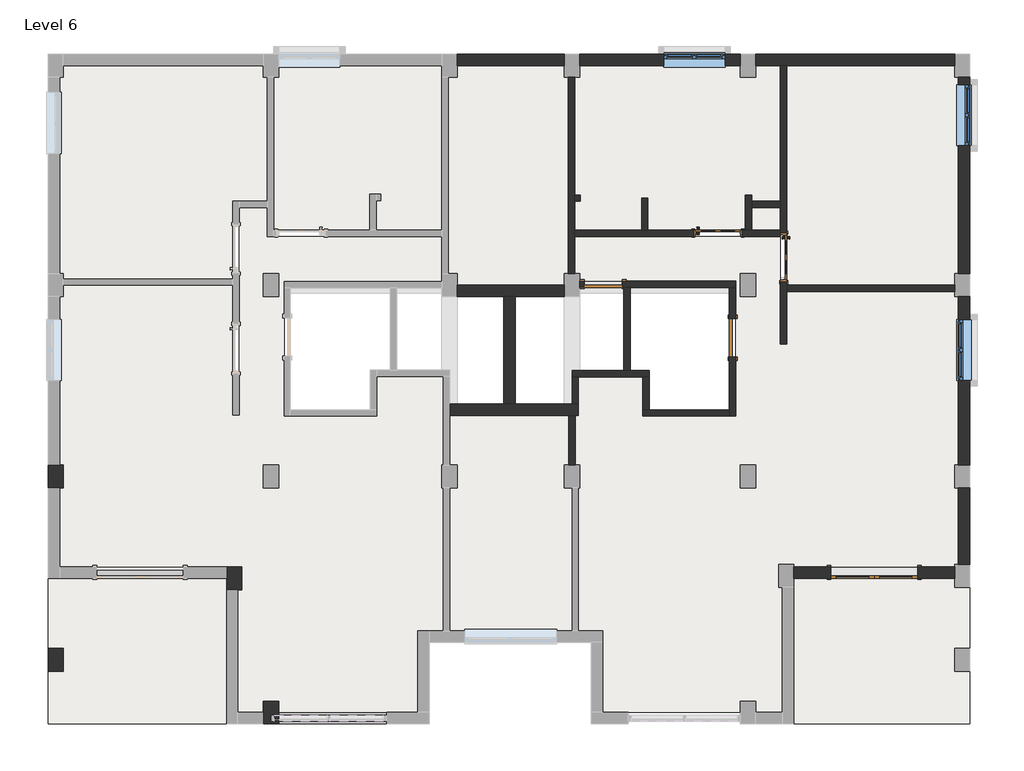
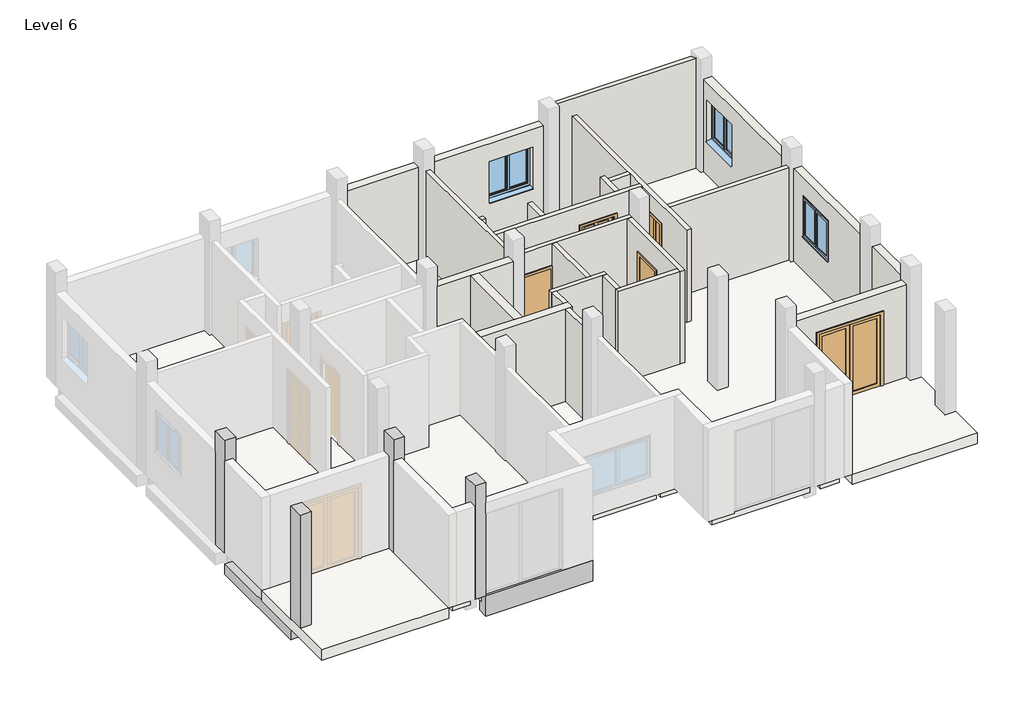
# One storey, part 2 of 3: 26 walls, 7 slabs, 5 doors, 4 columns, 3 beams, 3 windows.
"""IFC4 building model written with IfcOpenShell, lengths in millimetres."""

from ifc_helpers import new_model, si_unit, frame, origin, place, context, project, spatial, polyline, outline, extrude, faceted_brep, transform, mapped, element, save
from components import door_e52a3823, door_68a706ac, door_1fe7f57d, w2_0001_windows_4_x_4_9dec5fc7

model = new_model("IFC4")

# Units and contexts
model_context = context("Model", 3, world=origin())
ifc_project = project(units=[si_unit("LENGTHUNIT", "METRE", prefix="MILLI")], contexts=[model_context])

# Site, building, storey
site = spatial("IfcSite", under=ifc_project)
building = spatial("IfcBuilding", under=site)
storey = spatial("IfcBuildingStorey", under=building, Name="Level 6", Elevation=9448.8)

# Beams
placement = place(None, origin())
element("IfcBeam", 1, ObjectType="Concrete-Rectangular Beam : 12 x 24", at=placement, inside=storey, context=model_context, shape_type="Brep", body=[
    faceted_brep([(-9144.7786397, -9867.8620333, 8839.2), (-9144.7786397, -13068.2620333, 8839.2), (-9144.7786397, -13068.2620333, 9144.0), (-9144.7786397, -9867.8620333, 9144.0), (-8839.9786397, -9867.8620333, 8839.2), (-8839.9786397, -11518.8620333, 8839.2), (-8839.9786397, -11823.6620333, 8839.2), (-8839.9786397, -13068.2620333, 8839.2), (-8839.9786397, -9867.8620333, 9144.0), (-8839.9786397, -11518.8620333, 9144.0), (-8839.9786397, -11823.6620333, 9144.0), (-8839.9786397, -13068.2620333, 9144.0)], [[[0, 1, 2, 3]], [[1, 0, 4, 5, 6, 7]], [[7, 6, 5, 4, 8, 9, 10, 11]], [[4, 0, 3, 8]], [[1, 7, 11, 2]], [[3, 2, 11, 10, 9, 8]]]),
])
element("IfcBeam", 2, ObjectType="Concrete-Rectangular Beam : 12 x 24", at=placement, inside=storey, context=model_context, shape_type="SweptSolid", body=[
    extrude(outline(polyline([(-1550.9175798, -14272.0402089), (-1550.9175798, -14576.8402089), (-4548.1175798, -14576.8402089), (-4548.1175798, -14272.0402089), (-1550.9175798, -14272.0402089)])), frame((0.0, 0.0, 8839.2), z_axis=(0.0, 0.0, 1.0), x_axis=(1.0, 0.0, 0.0)), (0.0, 0.0, 1.0), 609.6),
])
element("IfcBeam", 3, ObjectType="Concrete-Rectangular Beam : 12 x 24", at=placement, inside=storey, context=model_context, shape_type="SweptSolid", body=[
    extrude(outline(polyline([(-8839.9786397, -11518.8620333), (-5589.5175798, -11518.8620333), (-5589.5175798, -11823.6620333), (-8839.9786397, -11823.6620333), (-8839.9786397, -11518.8620333)])), frame((0.0, 0.0, 8839.2), z_axis=(0.0, 0.0, 1.0), x_axis=(1.0, 0.0, 0.0)), (0.0, 0.0, 1.0), 304.8),
])

# Columns
element("IfcColumn", 4, ObjectType="Concrete-Rectangular-Column : 1'6\" X 1' COLUMN", at=placement, inside=storey, context=model_context, shape_type="Brep", body=[
    faceted_brep([(-8839.9786397, -9410.6620333, 9448.8), (-8839.9786397, -9867.8620333, 9448.8), (-9144.7786397, -9867.8620333, 9448.8), (-9144.7786397, -9410.6620333, 9448.8), (-8839.9786397, -9410.6620333, 12801.6), (-8839.9786397, -9867.8620333, 12801.6), (-8839.9786397, -9867.8620333, 9753.6), (-8839.9786397, -9410.6620333, 9753.6), (-9144.7786397, -9867.8620333, 12801.6), (-9144.7786397, -9867.8620333, 9753.6), (-9144.7786397, -9410.6620333, 12801.6), (-9144.7786397, -9410.6620333, 9753.6)], [[[0, 1, 2, 3]], [[4, 5, 6, 1, 0, 7]], [[5, 8, 9, 2, 1, 6]], [[8, 10, 11, 3, 2, 9]], [[10, 4, 7, 0, 3, 11]], [[4, 10, 8, 5]]]),
])
element("IfcColumn", 5, ObjectType="Concrete-Rectangular-Column : 1'6\" X 1' COLUMN", at=placement, inside=storey, context=model_context, shape_type="Brep", body=[
    faceted_brep([(-4548.1175798, -14119.6402089, 9448.8), (-4548.1175798, -14576.8402089, 9448.8), (-4852.9175798, -14576.8402089, 9448.8), (-4852.9175798, -14119.6402089, 9448.8), (-4548.1175798, -14119.6402089, 12801.6), (-4548.1175798, -14576.8402089, 12801.6), (-4548.1175798, -14119.6402089, 9753.6), (-4852.9175798, -14576.8402089, 12801.6), (-4852.9175798, -14119.6402089, 12801.6), (-4852.9175798, -14119.6402089, 9753.6)], [[[0, 1, 2, 3]], [[4, 5, 1, 0, 6]], [[5, 7, 2, 1]], [[7, 8, 9, 3, 2]], [[8, 4, 6, 0, 3, 9]], [[4, 8, 7, 5]]]),
])
element("IfcColumn", 6, ObjectType="Concrete-Rectangular-Column : 1'6\" X 1' COLUMN", at=placement, inside=storey, context=model_context, shape_type="Brep", body=[
    faceted_brep([(-8839.9786397, -13068.2620333, 9448.8), (-8839.9786397, -13525.4620333, 9448.8), (-9144.7786397, -13525.4620333, 9448.8), (-9144.7786397, -13068.2620333, 9448.8), (-8839.9786397, -13068.2620333, 12801.6), (-8839.9786397, -13525.4620333, 12801.6), (-8839.9786397, -13068.2620333, 9753.6), (-9144.7786397, -13525.4620333, 12801.6), (-9144.7786397, -13068.2620333, 12801.6), (-9144.7786397, -13068.2620333, 9753.6)], [[[0, 1, 2, 3]], [[4, 5, 1, 0, 6]], [[5, 7, 2, 1]], [[7, 8, 9, 3, 2]], [[8, 4, 6, 0, 3, 9]], [[4, 8, 7, 5]]]),
])
element("IfcColumn", 7, ObjectType="Concrete-Rectangular-Column : 1'6\" X 1' COLUMN", at=placement, inside=storey, context=model_context, shape_type="SweptSolid", body=[
    extrude(outline(polyline([(-5284.7175798, -11442.6620333), (-5284.7175798, -11899.8620333), (-5589.5175798, -11899.8620333), (-5589.5175798, -11442.6620333), (-5284.7175798, -11442.6620333)])), frame((0.0, 0.0, 9448.8), z_axis=(0.0, 0.0, 1.0), x_axis=(1.0, 0.0, 0.0)), (0.0, 0.0, 1.0), 3352.8),
])

# Doors
door_shape = door_e52a3823(model_context)
element("IfcDoor", 8, ObjectType="Door-Double-Glass : 68\" x 84\"", at=placement, inside=storey, context=model_context, shape_type="MappedRepresentation", body=[
    mapped(door_shape, transform((7313.6824202, -11554.5807833, 9448.8), x_axis=(-1.0, 0.0, 0.0), y_axis=(0.0, -1.0, 0.0), z_axis=(0.0, 0.0, 1.0))),
])
door_2_shape = door_68a706ac(model_context)
element("IfcDoor", 9, ObjectType="Door-Interior-Single-4_Panel-Wood : 36\" x 84\"", at=placement, inside=storey, context=model_context, shape_type="MappedRepresentation", body=[
    mapped(door_2_shape, transform((4202.1824202, -4789.1311634, 9448.8), x_axis=(1.0, 0.0, 0.0), y_axis=(0.0, 1.0, 0.0), z_axis=(0.0, 0.0, 1.0))),
])
element("IfcDoor", 10, ObjectType="Door-Interior-Single-4_Panel-Wood : 36\" x 84\"", at=placement, inside=storey, context=model_context, shape_type="MappedRepresentation", body=[
    mapped(door_2_shape, transform((5513.4574202, -5274.9061634, 9448.8), x_axis=(0.0, -1.0, 0.0), y_axis=(1.0, 0.0, 0.0), z_axis=(0.0, 0.0, 1.0))),
])
door_3_shape = door_1fe7f57d(model_context)
element("IfcDoor", 11, ObjectType="Single-Flush : 30\" x 80\"", at=placement, inside=storey, context=model_context, shape_type="MappedRepresentation", body=[
    mapped(door_3_shape, transform((1916.1824202, -5810.8691591, 9448.8), x_axis=(-1.0, 0.0, 0.0), y_axis=(0.0, -1.0, 0.0), z_axis=(0.0, 0.0, 1.0))),
])
element("IfcDoor", 12, ObjectType="Single-Flush : 30\" x 80\"", at=placement, inside=storey, context=model_context, shape_type="MappedRepresentation", body=[
    mapped(door_3_shape, transform((4494.2824202, -6877.6691591, 9448.8), x_axis=(0.0, 1.0, 0.0), y_axis=(-1.0, 0.0, 0.0), z_axis=(0.0, 0.0, 1.0))),
])

# Slabs
element("IfcSlab", 13, ObjectType="flooring 1'", at=placement, inside=storey, context=model_context, shape_type="SweptSolid", body=[
    extrude(outline(polyline([(-8916.1786397, -11442.6620333), (-8916.1786397, -9867.8620333), (-8839.9786397, -9867.8620333), (-8839.9786397, -9410.6620333), (-8916.1786397, -9410.6620333), (-8916.1786397, -6057.8620333), (-8839.9786397, -6057.8620333), (-8839.9786397, -5829.2620333), (-5462.5175798, -5829.2620333), (-5462.5175798, -8420.0620333), (-5335.5175798, -8420.0620333), (-5335.5175798, -4280.3104011), (-4776.7175798, -4280.3104011), (-4776.7175798, -4855.8061634), (-1296.9175798, -4855.8061634), (-1296.9175798, -5600.6620333), (-1296.9175798, -5758.8942903), (-4442.5950401, -5758.8942903), (-4442.5950401, -8439.1120333), (-2601.0950401, -8439.1120333), (-2601.0950401, -7651.7120333), (-1271.5175798, -7651.7120333), (-1271.5175798, -9410.6620333), (-1296.9175798, -9410.6620333), (-1296.9175798, -9867.8620333), (-1271.5175798, -9867.8620333), (-1271.5175798, -12722.6402089), (-1779.5175798, -12722.6402089), (-1779.5175798, -14348.2402089), (-4548.1175798, -14348.2402089), (-4548.1175798, -14119.6402089), (-4852.9175798, -14119.6402089), (-4852.9175798, -14348.2402089), (-5360.9175798, -14348.2402089), (-5360.9175798, -11899.8620333), (-5284.7175798, -11899.8620333), (-5284.7175798, -11442.6620333), (-5589.5175798, -11442.6620333), (-8916.1786397, -11442.6620333)])), frame((0.0, 0.0, 9144.0), z_axis=(0.0, 0.0, 1.0), x_axis=(1.0, 0.0, 0.0)), (0.0, 0.0, 1.0), 304.8),
])
element("IfcSlab", 14, ObjectType="flooring 1'", at=placement, inside=storey, context=model_context, shape_type="SweptSolid", body=[
    extrude(outline(polyline([(5446.7824202, -4855.8061634), (5446.7824202, -6583.0061634), (5573.7824202, -6583.0061634), (5573.7824202, -5956.2620333), (8913.8824202, -5956.2620333), (8913.8824202, -6057.8620333), (8990.0824202, -6057.8620333), (8990.0824202, -9410.6620333), (8913.8824202, -9410.6620333), (8913.8824202, -9867.8620333), (8990.0824202, -9867.8620333), (8990.0824202, -11391.8620333), (8913.8824202, -11391.8620333), (8913.8824202, -11442.6620333), (5713.4824202, -11442.6620333), (5713.4824202, -11391.8620333), (5408.6824202, -11391.8620333), (5408.6824202, -11849.0620333), (5484.8824202, -11849.0620333), (5484.8824202, -14348.2402089), (4951.4824202, -14348.2402089), (4951.4824202, -14119.6402089), (4646.6824202, -14119.6402089), (4646.6824202, -14348.2402089), (1903.4824202, -14348.2402089), (1903.4824202, -12722.6402089), (1420.8824202, -12722.6402089), (1420.8824202, -9867.8620333), (1446.2824202, -9867.8620333), (1446.2824202, -9410.6620333), (1357.3824202, -9410.6620333), (1357.3824202, -8426.4120333), (1420.8824202, -8426.4120333), (1420.8824202, -7660.8890971), (2703.5824202, -7660.8890971), (2703.5824202, -8439.7691591), (4557.7824202, -8439.7691591), (4557.7824202, -5747.3691591), (1446.2824202, -5747.3691591), (1446.2824202, -5600.6620333), (1344.6824202, -5600.6620333), (1344.6824202, -4855.8061634), (5446.7824202, -4855.8061634)])), frame((0.0, 0.0, 9144.0), z_axis=(0.0, 0.0, 1.0), x_axis=(1.0, 0.0, 0.0)), (0.0, 0.0, 1.0), 304.8),
])
element("IfcSlab", 15, ObjectType="flooring 1'", at=placement, inside=storey, context=model_context, shape_type="SweptSolid", body=[
    extrude(outline(polyline([(-8839.9786397, -1680.8061634), (-8839.9786397, -1452.2061634), (-4852.9175798, -1452.2061634), (-4852.9175798, -1680.8061634), (-4776.7175798, -1680.8061634), (-4776.7175798, -4153.3104011), (-5462.5175798, -4153.3104011), (-5462.5175798, -5702.2620333), (-8839.9786397, -5702.2620333), (-8839.9786397, -5600.6620333), (-8916.1786397, -5600.6620333), (-8916.1786397, -1680.8061634), (-8839.9786397, -1680.8061634)])), frame((0.0, 0.0, 9144.0), z_axis=(0.0, 0.0, 1.0), x_axis=(1.0, 0.0, 0.0)), (0.0, 0.0, 1.0), 304.8),
    extrude(outline(polyline([(-2732.0175798, -4728.8061634), (-4649.7175798, -4728.8061634), (-4649.7175798, -1680.8061634), (-4548.1175798, -1680.8061634), (-4548.1175798, -1452.2061634), (-1296.9175798, -1452.2061634), (-1296.9175798, -4728.8061634), (-2605.0175798, -4728.8061634), (-2605.0175798, -4144.6061634), (-2516.1175798, -4144.6061634), (-2516.1175798, -4017.6061634), (-2732.0175798, -4017.6061634), (-2732.0175798, -4728.8061634)])), frame((0.0, 0.0, 9144.0), z_axis=(0.0, 0.0, 1.0), x_axis=(1.0, 0.0, 0.0)), (0.0, 0.0, 1.0), 304.8),
])
element("IfcSlab", 16, ObjectType="flooring 1'", at=placement, inside=storey, context=model_context, shape_type="SweptSolid", body=[
    extrude(outline(polyline([(4646.6824202, -1452.2061634), (4646.6824202, -1680.8061634), (4951.4824202, -1680.8061634), (4951.4824202, -1452.2061634), (5446.7824202, -1452.2061634), (5446.7824202, -4157.3061634), (4875.2824202, -4157.3061634), (4875.2824202, -4030.3061634), (4748.2824202, -4030.3061634), (4748.2824202, -4728.8061634), (2805.1824202, -4728.8061634), (2805.1824202, -4093.8061634), (2678.1824202, -4093.8061634), (2678.1824202, -4728.8061634), (1344.6824202, -4728.8061634), (1344.6824202, -4157.3061634), (1458.9824202, -4157.3061634), (1458.9824202, -4030.3061634), (1344.6824202, -4030.3061634), (1344.6824202, -1680.8061634), (1446.2824202, -1680.8061634), (1446.2824202, -1452.2061634), (4646.6824202, -1452.2061634)])), frame((0.0, 0.0, 9144.0), z_axis=(0.0, 0.0, 1.0), x_axis=(1.0, 0.0, 0.0)), (0.0, 0.0, 1.0), 304.8),
    extrude(outline(polyline([(5446.7824202, -4284.3061634), (5446.7824202, -4728.8061634), (4875.2824202, -4728.8061634), (4875.2824202, -4284.3061634), (5446.7824202, -4284.3061634)])), frame((0.0, 0.0, 9144.0), z_axis=(0.0, 0.0, 1.0), x_axis=(1.0, 0.0, 0.0)), (0.0, 0.0, 1.0), 304.8),
    extrude(outline(polyline([(8913.8824202, -5829.2620333), (5573.7824202, -5829.2620333), (5573.7824202, -1452.2061634), (8913.8824202, -1452.2061634), (8913.8824202, -1680.8061634), (8990.0824202, -1680.8061634), (8990.0824202, -5600.6620333), (8913.8824202, -5600.6620333), (8913.8824202, -5829.2620333)])), frame((0.0, 0.0, 9144.0), z_axis=(0.0, 0.0, 1.0), x_axis=(1.0, 0.0, 0.0)), (0.0, 0.0, 1.0), 304.8),
])
element("IfcSlab", 17, ObjectType="flooring 1'", at=placement, inside=storey, context=model_context, shape_type="SweptSolid", body=[
    extrude(outline(polyline([(1141.4824202, -1452.2061634), (1141.4824202, -1680.8061634), (1217.6824202, -1680.8061634), (1217.6824202, -5600.6620333), (1141.4824202, -5600.6620333), (1141.4824202, -5829.2620333), (-992.1175798, -5829.2620333), (-992.1175798, -5600.6620333), (-1169.9175798, -5600.6620333), (-1169.9175798, -1680.8061634), (-992.1175798, -1680.8061634), (-992.1175798, -1452.2061634), (1141.4824202, -1452.2061634)])), frame((0.0, 0.0, 9144.0), z_axis=(0.0, 0.0, 1.0), x_axis=(1.0, 0.0, 0.0)), (0.0, 0.0, 1.0), 304.8),
])
element("IfcSlab", 18, ObjectType="flooring 1'", at=placement, inside=storey, context=model_context, shape_type="SweptSolid", body=[
    extrude(outline(polyline([(1293.8824202, -12722.6402089), (-1144.5175798, -12722.6402089), (-1144.5175798, -9867.8620333), (-992.1175798, -9867.8620333), (-992.1175798, -9410.6620333), (-1144.5175798, -9410.6620333), (-1144.5175798, -8426.4120333), (1230.3824202, -8426.4120333), (1230.3824202, -9410.6620333), (1141.4824202, -9410.6620333), (1141.4824202, -9867.8620333), (1293.8824202, -9867.8620333), (1293.8824202, -12722.6402089)])), frame((0.0, 0.0, 9144.0), z_axis=(0.0, 0.0, 1.0), x_axis=(1.0, 0.0, 0.0)), (0.0, 0.0, 1.0), 304.8),
])
element("IfcSlab", 19, ObjectType="flooring 1'", at=placement, inside=storey, context=model_context, shape_type="SweptSolid", body=[
    extrude(outline(polyline([(-5589.5175798, -11671.2620333), (-5589.5175798, -14576.8402089), (-9144.7786397, -14576.8402089), (-9144.7786397, -11671.2620333), (-5589.5175798, -11671.2620333)])), frame((0.0, 0.0, 9144.0), z_axis=(0.0, 0.0, 1.0), x_axis=(1.0, 0.0, 0.0)), (0.0, 0.0, 1.0), 304.8),
    extrude(outline(polyline([(9218.6824202, -11671.2620333), (9218.6824202, -14576.8402089), (5713.4824202, -14576.8402089), (5713.4824202, -11671.2620333), (9218.6824202, -11671.2620333)])), frame((0.0, 0.0, 9144.0), z_axis=(0.0, 0.0, 1.0), x_axis=(1.0, 0.0, 0.0)), (0.0, 0.0, 1.0), 304.8),
])

# Walls
element("IfcWall", 20, ObjectType="EXTERIOR WALL 9\"", at=placement, inside=storey, context=model_context, shape_type="SweptSolid", body=[
    extrude(outline(polyline([(1141.4824202, -1452.2061634), (-992.1175798, -1452.2061634), (-992.1175798, -1223.6061634), (1141.4824202, -1223.6061634), (1141.4824202, -1452.2061634)])), frame((0.0, 0.0, 9448.8), z_axis=(0.0, 0.0, 1.0), x_axis=(1.0, 0.0, 0.0)), (0.0, 0.0, 1.0), 2743.2),
])
element("IfcWall", 21, ObjectType="EXTERIOR WALL 9\"", at=placement, inside=storey, context=model_context, shape_type="SweptSolid", body=[
    extrude(outline(polyline([(9448.8, 1446.2824202), (9448.8, 4646.6824202), (12192.0, 4646.6824202), (12192.0, 1446.2824202), (9448.8, 1446.2824202)]), holes=[polyline([(10448.8, 4341.8824202), (10448.8, 3122.6824202), (11668.0, 3122.6824202), (11668.0, 4341.8824202), (10448.8, 4341.8824202)])]), frame((0.0, -1452.2061634, 0.0), z_axis=(0.0, 1.0, 0.0), x_axis=(0.0, 0.0, 1.0)), (0.0, 0.0, 1.0), 228.6),
])
element("IfcWall", 22, ObjectType="EXTERIOR WALL 9\"", at=placement, inside=storey, context=model_context, shape_type="Brep", body=[
    faceted_brep([(4951.4824202, -1452.2061634, 9448.8), (5446.7824202, -1452.2061634, 9448.8), (5573.7824202, -1452.2061634, 9448.8), (8913.8824202, -1452.2061634, 9448.8), (8913.8824202, -1452.2061634, 12704.6626409), (4951.4824202, -1452.2061634, 12704.6626409), (4951.4824202, -1223.6061634, 9448.8), (4951.4824202, -1223.6061634, 12615.578652), (8913.8824202, -1223.6061634, 12615.578652), (8913.8824202, -1223.6061634, 9448.8)], [[[0, 1, 2, 3, 4, 5]], [[6, 7, 8, 9]], [[3, 2, 1, 0, 6, 9]], [[4, 3, 9, 8]], [[0, 5, 7, 6]], [[5, 4, 8, 7]]]),
])
element("IfcWall", 23, ObjectType="EXTERIOR WALL 9\"", at=placement, inside=storey, context=model_context, shape_type="SweptSolid", body=[
    extrude(outline(polyline([(-1680.8061634, 9448.8), (-5600.6620333, 9448.8), (-5600.6620333, 12192.0), (-1680.8061634, 12192.0), (-1680.8061634, 9448.8)]), holes=[polyline([(-3052.4061634, 10448.8), (-1833.2061634, 10448.8), (-1833.2061634, 11668.0), (-3052.4061634, 11668.0), (-3052.4061634, 10448.8)])]), frame((8990.0824202, 0.0, 0.0), z_axis=(1.0, 0.0, 0.0), x_axis=(0.0, 1.0, 0.0)), (0.0, 0.0, 1.0), 228.6),
])
element("IfcWall", 24, ObjectType="EXTERIOR WALL 9\"", at=placement, inside=storey, context=model_context, shape_type="SweptSolid", body=[
    extrude(outline(polyline([(-6057.8620333, 9448.8), (-9410.6620333, 9448.8), (-9410.6620333, 12192.0), (-6057.8620333, 12192.0), (-6057.8620333, 9448.8)]), holes=[polyline([(-6515.0620333, 10448.8), (-6515.0620333, 11668.0), (-7734.2620333, 11668.0), (-7734.2620333, 10448.8), (-6515.0620333, 10448.8)])]), frame((8990.0824202, 0.0, 0.0), z_axis=(1.0, 0.0, 0.0), x_axis=(0.0, 1.0, 0.0)), (0.0, 0.0, 1.0), 228.6),
])
element("IfcWall", 25, ObjectType="EXTERIOR WALL 9\"", at=placement, inside=storey, context=model_context, shape_type="SweptSolid", body=[
    extrude(outline(polyline([(8990.0824202, -11391.8620333), (8990.0824202, -9867.8620333), (9218.6824202, -9867.8620333), (9218.6824202, -11391.8620333), (8990.0824202, -11391.8620333)])), frame((0.0, 0.0, 9448.8), z_axis=(0.0, 0.0, 1.0), x_axis=(1.0, 0.0, 0.0)), (0.0, 0.0, 1.0), 2743.2),
])
element("IfcWall", 26, ObjectType="EXTERIOR WALL 9\"", at=placement, inside=storey, context=model_context, shape_type="SweptSolid", body=[
    extrude(outline(polyline([(12192.0, 5713.4824202), (9448.8, 5713.4824202), (9448.8, 6450.0824202), (11582.4, 6450.0824202), (11582.4, 8177.2824202), (9448.8, 8177.2824202), (9448.8, 8913.8824202), (12192.0, 8913.8824202), (12192.0, 5713.4824202)])), frame((0.0, -11671.2620333, 0.0), z_axis=(0.0, 1.0, 0.0), x_axis=(0.0, 0.0, 1.0)), (0.0, 0.0, 1.0), 228.6),
])
element("IfcWall", 27, ObjectType="EXTERIOR WALL 9\"", at=placement, inside=storey, context=model_context, shape_type="Brep", body=[
    faceted_brep([(1141.4824202, -5829.2620333, 9448.8), (-992.1175798, -5829.2620333, 9448.8), (-992.1175798, -5829.2620333, 12192.0), (1141.4824202, -5829.2620333, 12192.0), (1141.4824202, -6057.8620333, 9448.8), (1141.4824202, -6057.8620333, 12192.0), (163.5824202, -6057.8620333, 12192.0), (-65.0175798, -6057.8620333, 12192.0), (-992.1175798, -6057.8620333, 12192.0), (-992.1175798, -6057.8620333, 9448.8), (-65.0175798, -6057.8620333, 9448.8), (163.5824202, -6057.8620333, 9448.8)], [[[0, 1, 2, 3]], [[4, 5, 6, 7, 8, 9, 10, 11]], [[1, 0, 4, 11, 10, 9]], [[2, 1, 9, 8]], [[3, 2, 8, 7, 6, 5]], [[0, 3, 5, 4]]]),
])
element("IfcWall", 28, ObjectType="EXTERIOR WALL 9\"", at=placement, inside=storey, context=model_context, shape_type="SweptSolid", body=[
    extrude(outline(polyline([(-65.0175798, -8197.8120333), (-65.0175798, -6057.8620333), (163.5824202, -6057.8620333), (163.5824202, -8197.8120333), (-65.0175798, -8197.8120333)])), frame((0.0, 0.0, 9448.8), z_axis=(0.0, 0.0, 1.0), x_axis=(1.0, 0.0, 0.0)), (0.0, 0.0, 1.0), 2743.2),
])
element("IfcWall", 29, ObjectType="EXTERIOR WALL 9\"", at=placement, inside=storey, context=model_context, shape_type="Brep", body=[
    faceted_brep([(-1144.5175798, -8426.4120333, 9448.8), (1230.3824202, -8426.4120333, 9448.8), (1357.3824202, -8426.4120333, 9448.8), (1420.8824202, -8426.4120333, 9448.8), (1420.8824202, -8426.4120333, 12192.0), (1357.3824202, -8426.4120333, 12192.0), (1230.3824202, -8426.4120333, 12192.0), (-1144.5175798, -8426.4120333, 12192.0), (-1144.5175798, -8197.8120333, 9448.8), (-1144.5175798, -8197.8120333, 12192.0), (-65.0175798, -8197.8120333, 12192.0), (163.5824202, -8197.8120333, 12192.0), (1293.8824202, -8197.8120333, 12192.0), (1420.8824202, -8197.8120333, 12192.0), (1420.8824202, -8197.8120333, 9448.8), (1293.8824202, -8197.8120333, 9448.8), (163.5824202, -8197.8120333, 9448.8), (-65.0175798, -8197.8120333, 9448.8)], [[[0, 1, 2, 3, 4, 5, 6, 7]], [[8, 9, 10, 11, 12, 13, 14, 15, 16, 17]], [[3, 2, 1, 0, 8, 17, 16, 15, 14]], [[7, 6, 5, 4, 13, 12, 11, 10, 9]], [[0, 7, 9, 8]], [[4, 3, 14, 13]]]),
])
element("IfcWall", 30, ObjectType="INTERIOR WALL 5\"", at=placement, inside=storey, context=model_context, shape_type="Brep", body=[
    faceted_brep([(1217.6824202, -1680.8061634, 9448.8), (1217.6824202, -5600.6620333, 9448.8), (1217.6824202, -5600.6620333, 12192.0), (1217.6824202, -1680.8061634, 12192.0), (1344.6824202, -1680.8061634, 9448.8), (1344.6824202, -1680.8061634, 12192.0), (1344.6824202, -4030.3061634, 12192.0), (1344.6824202, -4157.3061634, 12192.0), (1344.6824202, -4728.8061634, 12192.0), (1344.6824202, -4855.8061634, 12192.0), (1344.6824202, -5600.6620333, 12192.0), (1344.6824202, -5600.6620333, 9448.8), (1344.6824202, -4855.8061634, 9448.8), (1344.6824202, -4728.8061634, 9448.8), (1344.6824202, -4157.3061634, 9448.8), (1344.6824202, -4030.3061634, 9448.8)], [[[0, 1, 2, 3]], [[4, 5, 6, 7, 8, 9, 10, 11, 12, 13, 14, 15]], [[1, 0, 4, 15, 14, 13, 12, 11]], [[2, 1, 11, 10]], [[3, 2, 10, 9, 8, 7, 6, 5]], [[0, 3, 5, 4]]]),
])
element("IfcWall", 31, ObjectType="INTERIOR WALL 5\"", at=placement, inside=storey, context=model_context, shape_type="Brep", body=[
    faceted_brep([(5446.7824202, -4855.8061634, 12192.0), (1344.6824202, -4855.8061634, 12192.0), (1344.6824202, -4855.8061634, 9448.8), (3719.5824202, -4855.8061634, 9448.8), (3719.5824202, -4855.8061634, 11607.8), (4684.7824202, -4855.8061634, 11607.8), (4684.7824202, -4855.8061634, 9448.8), (5446.7824202, -4855.8061634, 9448.8), (1344.6824202, -4728.8061634, 12192.0), (2678.1824202, -4728.8061634, 12192.0), (2805.1824202, -4728.8061634, 12192.0), (4748.2824202, -4728.8061634, 12192.0), (4875.2824202, -4728.8061634, 12192.0), (5446.7824202, -4728.8061634, 12192.0), (5446.7824202, -4728.8061634, 9448.8), (4875.2824202, -4728.8061634, 9448.8), (4748.2824202, -4728.8061634, 9448.8), (4684.7824202, -4728.8061634, 9448.8), (4684.7824202, -4728.8061634, 11607.8), (3719.5824202, -4728.8061634, 11607.8), (3719.5824202, -4728.8061634, 9448.8), (2805.1824202, -4728.8061634, 9448.8), (2678.1824202, -4728.8061634, 9448.8), (1344.6824202, -4728.8061634, 9448.8)], [[[0, 1, 2, 3, 4, 5, 6, 7]], [[8, 9, 10, 11, 12, 13, 14, 15, 16, 17, 18, 19, 20, 21, 22, 23]], [[2, 23, 22, 21, 20, 3]], [[14, 7, 6, 17, 16, 15]], [[1, 0, 13, 12, 11, 10, 9, 8]], [[2, 1, 8, 23]], [[0, 7, 14, 13]], [[5, 18, 17, 6]], [[18, 5, 4, 19]], [[19, 4, 3, 20]]]),
])
element("IfcWall", 32, ObjectType="INTERIOR WALL 5\"", at=placement, inside=storey, context=model_context, shape_type="Brep", body=[
    faceted_brep([(4875.2824202, -4728.8061634, 9448.8), (4875.2824202, -4284.3061634, 9448.8), (4875.2824202, -4157.3061634, 9448.8), (4875.2824202, -4030.3061634, 9448.8), (4875.2824202, -4030.3061634, 12192.0), (4875.2824202, -4157.3061634, 12192.0), (4875.2824202, -4284.3061634, 12192.0), (4875.2824202, -4728.8061634, 12192.0), (4748.2824202, -4728.8061634, 9448.8), (4748.2824202, -4728.8061634, 12192.0), (4748.2824202, -4030.3061634, 12192.0), (4748.2824202, -4030.3061634, 9448.8)], [[[0, 1, 2, 3, 4, 5, 6, 7]], [[8, 9, 10, 11]], [[3, 2, 1, 0, 8, 11]], [[4, 3, 11, 10]], [[7, 6, 5, 4, 10, 9]], [[0, 7, 9, 8]]]),
])
element("IfcWall", 33, ObjectType="INTERIOR WALL 5\"", at=placement, inside=storey, context=model_context, shape_type="SweptSolid", body=[
    extrude(outline(polyline([(5446.7824202, -4284.3061634), (4875.2824202, -4284.3061634), (4875.2824202, -4157.3061634), (5446.7824202, -4157.3061634), (5446.7824202, -4284.3061634)])), frame((0.0, 0.0, 9448.8), z_axis=(0.0, 0.0, 1.0), x_axis=(1.0, 0.0, 0.0)), (0.0, 0.0, 1.0), 2743.2),
])
element("IfcWall", 34, ObjectType="INTERIOR WALL 5\"", at=placement, inside=storey, context=model_context, shape_type="Brep", body=[
    faceted_brep([(5446.7824202, -7002.1061634, 9448.8), (5446.7824202, -7002.1061634, 12192.0), (5446.7824202, -4855.8061634, 12192.0), (5446.7824202, -4728.8061634, 12192.0), (5446.7824202, -4284.3061634, 12192.0), (5446.7824202, -4157.3061634, 12192.0), (5446.7824202, -1452.2061634, 12192.0), (5446.7824202, -1452.2061634, 9448.8), (5446.7824202, -4157.3061634, 9448.8), (5446.7824202, -4284.3061634, 9448.8), (5446.7824202, -4728.8061634, 9448.8), (5446.7824202, -4792.3061634, 9448.8), (5446.7824202, -4792.3061634, 11607.8), (5446.7824202, -5757.5061634, 11607.8), (5446.7824202, -5757.5061634, 9448.8), (5573.7824202, -7002.1061634, 12192.0), (5573.7824202, -7002.1061634, 9448.8), (5573.7824202, -5956.2620333, 9448.8), (5573.7824202, -5829.2620333, 9448.8), (5573.7824202, -5757.5061634, 9448.8), (5573.7824202, -5757.5061634, 11607.8), (5573.7824202, -4792.3061634, 11607.8), (5573.7824202, -4792.3061634, 9448.8), (5573.7824202, -1452.2061634, 9448.8), (5573.7824202, -1452.2061634, 12192.0), (5573.7824202, -5829.2620333, 12192.0), (5573.7824202, -5956.2620333, 12192.0)], [[[0, 1, 2, 3, 4, 5, 6, 7, 8, 9, 10, 11, 12, 13, 14]], [[15, 16, 17, 18, 19, 20, 21, 22, 23, 24, 25, 26]], [[16, 0, 14, 19, 18, 17]], [[7, 23, 22, 11, 10, 9, 8]], [[1, 0, 16, 15]], [[6, 5, 4, 3, 2, 1, 15, 26, 25, 24]], [[7, 6, 24, 23]], [[13, 20, 19, 14]], [[20, 13, 12, 21]], [[21, 12, 11, 22]]]),
])
element("IfcWall", 35, ObjectType="INTERIOR WALL 5\"", at=placement, inside=storey, context=model_context, shape_type="SweptSolid", body=[
    extrude(outline(polyline([(5573.7824202, -5829.2620333), (8913.8824202, -5829.2620333), (8913.8824202, -5956.2620333), (5573.7824202, -5956.2620333), (5573.7824202, -5829.2620333)])), frame((0.0, 0.0, 9448.8), z_axis=(0.0, 0.0, 1.0), x_axis=(1.0, 0.0, 0.0)), (0.0, 0.0, 1.0), 2743.2),
])
element("IfcWall", 36, ObjectType="INTERIOR WALL 5\"", at=placement, inside=storey, context=model_context, shape_type="SweptSolid", body=[
    extrude(outline(polyline([(2805.1824202, -4093.8061634), (2805.1824202, -4728.8061634), (2678.1824202, -4728.8061634), (2678.1824202, -4093.8061634), (2805.1824202, -4093.8061634)])), frame((0.0, 0.0, 9448.8), z_axis=(0.0, 0.0, 1.0), x_axis=(1.0, 0.0, 0.0)), (0.0, 0.0, 1.0), 2743.2),
])
element("IfcWall", 37, ObjectType="INTERIOR WALL 5\"", at=placement, inside=storey, context=model_context, shape_type="SweptSolid", body=[
    extrude(outline(polyline([(1458.9824202, -4157.3061634), (1344.6824202, -4157.3061634), (1344.6824202, -4030.3061634), (1458.9824202, -4030.3061634), (1458.9824202, -4157.3061634)])), frame((0.0, 0.0, 9448.8), z_axis=(0.0, 0.0, 1.0), x_axis=(1.0, 0.0, 0.0)), (0.0, 0.0, 1.0), 2743.2),
])
element("IfcWall", 38, ObjectType="INTERIOR WALL 5\"", at=placement, inside=storey, context=model_context, shape_type="Brep", body=[
    faceted_brep([(1535.1824202, -5747.3691591, 11480.8), (1535.1824202, -5747.3691591, 9448.8), (1446.2824202, -5747.3691591, 9448.8), (1446.2824202, -5747.3691591, 12192.0), (4557.7824202, -5747.3691591, 12192.0), (4557.7824202, -5747.3691591, 9448.8), (2297.1824202, -5747.3691591, 9448.8), (2297.1824202, -5747.3691591, 11480.8), (1446.2824202, -5874.3691591, 9448.8), (1535.1824202, -5874.3691591, 9448.8), (1535.1824202, -5874.3691591, 11480.8), (2297.1824202, -5874.3691591, 11480.8), (2297.1824202, -5874.3691591, 9448.8), (2322.5824202, -5874.3691591, 9448.8), (2449.5824202, -5874.3691591, 9448.8), (4430.7824202, -5874.3691591, 9448.8), (4557.7824202, -5874.3691591, 9448.8), (4557.7824202, -5874.3691591, 12192.0), (4430.7824202, -5874.3691591, 12192.0), (2449.5824202, -5874.3691591, 12192.0), (2322.5824202, -5874.3691591, 12192.0), (1446.2824202, -5874.3691591, 12192.0)], [[[0, 1, 2, 3, 4, 5, 6, 7]], [[8, 9, 10, 11, 12, 13, 14, 15, 16, 17, 18, 19, 20, 21]], [[6, 5, 16, 15, 14, 13, 12]], [[2, 1, 9, 8]], [[3, 2, 8, 21]], [[4, 3, 21, 20, 19, 18, 17]], [[5, 4, 17, 16]], [[10, 9, 1, 0]], [[11, 10, 0, 7]], [[12, 11, 7, 6]]]),
])
element("IfcWall", 39, ObjectType="INTERIOR WALL 5\"", at=placement, inside=storey, context=model_context, shape_type="Brep", body=[
    faceted_brep([(4430.7824202, -5874.3691591, 9448.8), (4430.7824202, -6496.6691591, 9448.8), (4430.7824202, -6496.6691591, 11480.8), (4430.7824202, -7258.6691591, 11480.8), (4430.7824202, -7258.6691591, 9448.8), (4430.7824202, -8312.7691591, 9448.8), (4430.7824202, -8439.7691591, 9448.8), (4430.7824202, -8439.7691591, 12192.0), (4430.7824202, -8312.7691591, 12192.0), (4430.7824202, -5874.3691591, 12192.0), (4557.7824202, -6496.6691591, 11480.8), (4557.7824202, -6496.6691591, 9448.8), (4557.7824202, -5874.3691591, 9448.8), (4557.7824202, -5874.3691591, 12192.0), (4557.7824202, -8439.7691591, 12192.0), (4557.7824202, -8439.7691591, 9448.8), (4557.7824202, -7258.6691591, 9448.8), (4557.7824202, -7258.6691591, 11480.8)], [[[0, 1, 2, 3, 4, 5, 6, 7, 8, 9]], [[10, 11, 12, 13, 14, 15, 16, 17]], [[16, 15, 6, 5, 4]], [[12, 11, 1, 0]], [[9, 8, 7, 14, 13]], [[0, 9, 13, 12]], [[7, 6, 15, 14]], [[2, 1, 11, 10]], [[3, 2, 10, 17]], [[4, 3, 17, 16]]]),
])
element("IfcWall", 40, ObjectType="INTERIOR WALL 5\"", at=placement, inside=storey, context=model_context, shape_type="Brep", body=[
    faceted_brep([(4430.7824202, -8312.7691591, 9448.8), (2830.5824202, -8312.7691591, 9448.8), (2703.5824202, -8312.7691591, 9448.8), (2703.5824202, -8312.7691591, 12192.0), (2830.5824202, -8312.7691591, 12192.0), (4430.7824202, -8312.7691591, 12192.0), (4430.7824202, -8439.7691591, 9448.8), (4430.7824202, -8439.7691591, 12192.0), (2703.5824202, -8439.7691591, 12192.0), (2703.5824202, -8439.7691591, 9448.8)], [[[0, 1, 2, 3, 4, 5]], [[6, 7, 8, 9]], [[2, 1, 0, 6, 9]], [[5, 4, 3, 8, 7]], [[0, 5, 7, 6]], [[3, 2, 9, 8]]]),
])
element("IfcWall", 41, ObjectType="INTERIOR WALL 5\"", at=placement, inside=storey, context=model_context, shape_type="SweptSolid", body=[
    extrude(outline(polyline([(2830.5824202, -7660.8890971), (2830.5824202, -8312.7691591), (2703.5824202, -8312.7691591), (2703.5824202, -7660.8890971), (2830.5824202, -7660.8890971)])), frame((0.0, 0.0, 9448.8), z_axis=(0.0, 0.0, 1.0), x_axis=(1.0, 0.0, 0.0)), (0.0, 0.0, 1.0), 2743.2),
])
element("IfcWall", 42, ObjectType="INTERIOR WALL 5\"", at=placement, inside=storey, context=model_context, shape_type="Brep", body=[
    faceted_brep([(2830.5824202, -7533.8890971, 9448.8), (2449.5824202, -7533.8890971, 9448.8), (2322.5824202, -7533.8890971, 9448.8), (1293.8824202, -7533.8890971, 9448.8), (1293.8824202, -7533.8890971, 12192.0), (2322.5824202, -7533.8890971, 12192.0), (2449.5824202, -7533.8890971, 12192.0), (2830.5824202, -7533.8890971, 12192.0), (2830.5824202, -7660.8890971, 9448.8), (2830.5824202, -7660.8890971, 12192.0), (2703.5824202, -7660.8890971, 12192.0), (1420.8824202, -7660.8890971, 12192.0), (1293.8824202, -7660.8890971, 12192.0), (1293.8824202, -7660.8890971, 9448.8), (1420.8824202, -7660.8890971, 9448.8), (2703.5824202, -7660.8890971, 9448.8)], [[[0, 1, 2, 3, 4, 5, 6, 7]], [[8, 9, 10, 11, 12, 13, 14, 15]], [[3, 2, 1, 0, 8, 15, 14, 13]], [[7, 6, 5, 4, 12, 11, 10, 9]], [[0, 7, 9, 8]], [[4, 3, 13, 12]]]),
])
element("IfcWall", 43, ObjectType="INTERIOR WALL 5\"", at=placement, inside=storey, context=model_context, shape_type="SweptSolid", body=[
    extrude(outline(polyline([(1293.8824202, -8197.8120333), (1293.8824202, -7660.8890971), (1420.8824202, -7660.8890971), (1420.8824202, -8197.8120333), (1293.8824202, -8197.8120333)])), frame((0.0, 0.0, 9448.8), z_axis=(0.0, 0.0, 1.0), x_axis=(1.0, 0.0, 0.0)), (0.0, 0.0, 1.0), 2743.2),
])
element("IfcWall", 44, ObjectType="INTERIOR WALL 5\"", at=placement, inside=storey, context=model_context, shape_type="SweptSolid", body=[
    extrude(outline(polyline([(2322.5824202, -7533.8890971), (2322.5824202, -5874.3691591), (2449.5824202, -5874.3691591), (2449.5824202, -7533.8890971), (2322.5824202, -7533.8890971)])), frame((0.0, 0.0, 9448.8), z_axis=(0.0, 0.0, 1.0), x_axis=(1.0, 0.0, 0.0)), (0.0, 0.0, 1.0), 2743.2),
])
element("IfcWall", 45, ObjectType="INTERIOR WALL 5\"", at=placement, inside=storey, context=model_context, shape_type="SweptSolid", body=[
    extrude(outline(polyline([(1357.3824202, -8426.4120333), (1357.3824202, -9410.6620333), (1230.3824202, -9410.6620333), (1230.3824202, -8426.4120333), (1357.3824202, -8426.4120333)])), frame((0.0, 0.0, 9448.8), z_axis=(0.0, 0.0, 1.0), x_axis=(1.0, 0.0, 0.0)), (0.0, 0.0, 1.0), 2743.2),
])

# Windows
w2_0001_windows_4_x_4_shape = w2_0001_windows_4_x_4_9dec5fc7(model_context)
element("IfcWindow", 46, ObjectType="w2.0001 : WINDOWS 4' X 4'", at=placement, inside=storey, context=model_context, shape_type="MappedRepresentation", body=[
    mapped(w2_0001_windows_4_x_4_shape, transform((9104.3824202, -7124.6620333, 9448.8), x_axis=(0.0, -1.0, 0.0), y_axis=(1.0, 0.0, 0.0), z_axis=(0.0, 0.0, 1.0))),
])
element("IfcWindow", 47, ObjectType="w2.0001 : WINDOWS 4' X 4'", at=placement, inside=storey, context=model_context, shape_type="MappedRepresentation", body=[
    mapped(w2_0001_windows_4_x_4_shape, transform((9104.3824202, -2442.8061634, 9448.8), x_axis=(0.0, 1.0, 0.0), y_axis=(-1.0, 0.0, 0.0), z_axis=(0.0, 0.0, 1.0))),
])
element("IfcWindow", 48, ObjectType="w2.0001 : WINDOWS 4' X 4'", at=placement, inside=storey, context=model_context, shape_type="MappedRepresentation", body=[
    mapped(w2_0001_windows_4_x_4_shape, transform((3732.2824202, -1337.9061634, 9448.8), x_axis=(-1.0, 0.0, 0.0), y_axis=(0.0, -1.0, 0.0), z_axis=(0.0, 0.0, 1.0))),
])

save(model, "model.ifc")

# Revit data of these elements
# Type "Concrete-Rectangular Beam : 12 x 24"
#   Assembly Code = "B10"
#   Length [instance default] = 5' - 0"
#   b = 1' - 0"
#   h = 2' - 0"
#   Structural Material [instance default] = Concrete, Cast-in-Place gray
# Type "Concrete-Rectangular-Column : 1'6\" X 1' COLUMN"
#   Assembly Code = "B10"
#   b = 1' - 0"
#   h = 1' - 6"
#   Structural Material [instance default] = Concrete, Cast-in-Place gray
# Type "Door-Double-Glass : 68\" x 84\""
#   Type Mark = "11"
#   Construction Type Id = "opn-d45"
#   Assembly Code = "C1020"
#   Analytic Construction = "Wood frame, double glass door "
#   W = 2' - 10"
#   Thickness = 0' - 2"
#   Thermal Resistance (R) = 1.8150 (h·ft²·°F)/BTU
#   Swing Angle [instance default] = 90.00°
#   Heat Transfer Coefficient (U) = 0.5510 BTU/(h·ft²·°F)
#   Height = 7' - 0"
#   Bottom Rail = 0' - 4"
#   Top Rail = 0' - 4"
#   Stiles = 0' - 4"
#   Trim Projection = 0' - 1"
#   Trim Width = 0' - 3"
#   Width = 5' - 8"
#   Define Thermal Properties by = 1
#   Glazing = Glass
#   Panel Material = Wood - Birch - Solid Stained Light Low Gloss
#   Trim Material = Paint - Sienna
#   Visual Light Transmittance = 0
#   Solar Heat Gain Coefficient = 0
#   Function = (empty or 0)
#   Wall Closure = (empty or 0)
# Type "Door-Interior-Single-4_Panel-Wood : 36\" x 84\""
#   Type Mark = "9"
#   Assembly Code = "C1020300"
#   Analytic Construction = "Wooden"
#   Top Rail = 0' - 4 11/16"
#   Thickness = 0' - 1 3/8"
#   Thermal Resistance (R) = 2.5876 (h·ft²·°F)/BTU
#   Swing Angle [instance default] = 90.00°
#   Stiles = 0' - 4 3/4"
#   Rough Width = 3' - 2"
#   Rough Height = 7' - 1"
#   Mullion = 0' - 4 1/2"
#   Lock Rail = 0' - 7 1/2"
#   Height = 7' - 0"
#   Width = 3' - 0"
#   Heat Transfer Coefficient (U) = 0.3865 BTU/(h·ft²·°F)
#   Bottom Rail = 0' - 9 1/8"
#   Trim Material = Cherry
#   Panel Material = Cherry
#   Frame Material = Cherry
#   Door Handle Material = Aluminum
#   Visual Light Transmittance = 0
#   Solar Heat Gain Coefficient = 0
#   Wall Closure = (empty or 0)
#   Function = (empty or 0)
# Type "Single-Flush : 30\" x 80\""
#   Type Mark = "5"
#   Construction Type Id = "MDOOR"
#   Assembly Code = "C1020"
#   Analytic Construction = "Metal"
#   Thickness = 0' - 2"
#   Heat Transfer Coefficient (U) = 0.651978 BTU/(h·ft²·°F)
#   Height = 6' - 8"
#   Trim Projection Ext = 0' - 1"
#   Trim Projection Int = 0' - 1"
#   Trim Width = 0' - 3"
#   Width = 2' - 6"
#   Define Thermal Properties by = 1
#   Define Thermal Properties by = 1
#   Door Material = Door - Panel
#   Frame Material = Door - Frame
#   Visual Light Transmittance = 0
#   Solar Heat Gain Coefficient = 0
#   Function = (empty or 0)
#   Wall Closure = (empty or 0)
# Type "flooring 1'"
#   Assembly Code = "B1010"
#   Function = 0
#   Layers, outside or top first: 1' - 0" "FL_MARBLE WHITE" (function 1)
# Type "EXTERIOR WALL 9\""
#   Assembly Code = "B2010"
#   Layers, outside or top first: 0' - 9" "WARM BEIGE COLOUR" (function 1)
# Type "INTERIOR WALL 5\""
#   Assembly Code = "B2010"
#   Layers, outside or top first: 0' - 5" "WARM BEIGE COLOUR" (function 1)
# Type "w2.0001 : WINDOWS 4' X 4'"
#   Type Mark = "21"
#   Operation = "DoublePanelVertical"
#   Keynote = "16.05.01"
#   Analytic Construction = "<None>"
#   Rough Width = 4' - 0"
#   Rough Height = 4' - 0"
#   Rahmentiefe = 0' - 2.3622"
#   Rahmenhöhe unten = 0' - 3.14961"
#   Rahmehöhe oben = 0' - 3.14961"
#   Rahmenbreite = 0' - 2.3622"
#   Height = 4' - 0"
#   Flügeltiefe = 0' - 2.3622"
#   Flügelbreite = 0' - 2.3622"
#   Einbautiefe (von außen) [instance default] = 0' - 5.51181"
#   Width = 4' - 0"
#   Kippflügel [instance default] = yes
#   Drehflügel im Grundriß darstellen [instance default] = no
#   Drehflügel [instance default] = yes
#   Define Thermal Properties by = 1
#   Rahmen [instance default] = none
#   Glas [instance default] = none
#   Flügel [instance default] = none
#   Fensterbank aussen [instance default] = none
#   Fensterbank innen [instance default] = none
#   Wall Closure = (empty or 0)
# Elements 1, 2, 3 (IfcBeam, "Concrete-Rectangular Beam : 12 x 24")
#   Structural Material = WARM BEIGE COLOUR
#   Phase Created = New Construction
#   Materials on its faces: "WARM BEIGE COLOUR"
# Elements 4, 5, 6, 7 (IfcColumn, "Concrete-Rectangular-Column : 1'6\" X 1' COLUMN")
#   Structural Material = WARM BEIGE COLOUR
#   Phase Created = New Construction
#   Materials on its faces: "WARM BEIGE COLOUR"
# Element 8 (IfcDoor, "Door-Double-Glass : 68\" x 84\"")
#   Phase Created = New Construction
#   Materials on its faces: "Wood - Birch - Solid Stained Light Low Gloss", "Paint - Sienna", "Glass"
# Elements 9, 10 (IfcDoor, "Door-Interior-Single-4_Panel-Wood : 36\" x 84\"")
#   Swing Angle = 90.00°
#   Phase Created = New Construction
#   Materials on its faces: "Cherry", "Aluminum"
# Elements 11, 12 (IfcDoor, "Single-Flush : 30\" x 80\"")
#   Phase Created = New Construction
#   Materials on its faces: "Door - Frame", "Door - Panel"
# Element 13 (IfcSlab, "flooring 1'")
#   built-in parameter 1001955 = 3.14159 (stored number, unit not read)
#   Height Offset From Level = 0' - 0"
#   Phase Created = New Construction
#   Materials on its faces: "FL_MARBLE WHITE"
# Elements 14, 16, 17, 18, 19 (IfcSlab, "flooring 1'")
#   Height Offset From Level = 0' - 0"
#   Phase Created = New Construction
#   Materials on its faces: "FL_MARBLE WHITE"
# Element 15 (IfcSlab, "flooring 1'")
#   built-in parameter 1001955 = -1.5708 (stored number, unit not read)
#   Height Offset From Level = 0' - 0"
#   Phase Created = New Construction
#   Materials on its faces: "FL_MARBLE WHITE"
# Elements 20, 21, 22, 23, 24, 25, 26, 27, 28, 29 (IfcWall, "EXTERIOR WALL 9\"")
#   Top Offset = 9' - 0"
#   Base Offset = 0' - 0"
#   wall height = 9' - 0"
#   Phase Created = New Construction
#   Base Constraint = Level 6
#   Top Constraint = Level 6
#   Materials on its faces: "WARM BEIGE COLOUR"
# Elements 30, 31, 32, 33, 34, 35, 36, 37, 38, 39, 40, 41, 42, 43, 44, 45 (IfcWall, "INTERIOR WALL 5\"")
#   Top Offset = 9' - 0"
#   Base Offset = 0' - 0"
#   wall height = 9' - 0"
#   Phase Created = New Construction
#   Base Constraint = Level 6
#   Top Constraint = Level 6
#   Materials on its faces: "WARM BEIGE COLOUR"
# Element 46 (IfcWindow, "w2.0001 : WINDOWS 4' X 4'")
#   Mark = "35"
#   Einbautiefe (von außen) = 0' - 5.51181"
#   Kippflügel = yes
#   Drehflügel im Grundriß darstellen = no
#   Drehflügel = yes
#   Rahmen = none
#   Glas = none
#   Flügel = none
#   Fensterbank innen = none
#   Fensterbank aussen = none
#   Phase Created = New Construction
#   Materials on its faces: "Fenster - Kunststoff", "Fenster - Kunststoff weiss", "Glass", "Fenster - Holz"
# Element 47 (IfcWindow, "w2.0001 : WINDOWS 4' X 4'")
#   Mark = "36"
#   Einbautiefe (von außen) = 0' - 5.51181"
#   Kippflügel = yes
#   Drehflügel im Grundriß darstellen = no
#   Drehflügel = yes
#   Rahmen = none
#   Glas = none
#   Flügel = none
#   Fensterbank innen = none
#   Fensterbank aussen = none
#   Phase Created = New Construction
#   Materials on its faces: "Fenster - Kunststoff", "Fenster - Kunststoff weiss", "Glass", "Fenster - Holz"
# Element 48 (IfcWindow, "w2.0001 : WINDOWS 4' X 4'")
#   Mark = "37"
#   Einbautiefe (von außen) = 0' - 5.51181"
#   Kippflügel = yes
#   Drehflügel im Grundriß darstellen = no
#   Drehflügel = yes
#   Rahmen = none
#   Glas = none
#   Flügel = none
#   Fensterbank innen = none
#   Fensterbank aussen = none
#   Phase Created = New Construction
#   Materials on its faces: "Fenster - Kunststoff", "Fenster - Kunststoff weiss", "Glass", "Fenster - Holz"
# Materials
#   "Concrete, Cast-in-Place gray": class "Concrete", colour RGB 192 192 192, transparency 0, Description = "Cast-in-place concrete", Cost = 0
#   "Glass": class "Glass", colour RGB 0 128 192, transparency 0.75, Description = "Soda Lime Glass", Cost = 0
#   "Wood - Birch - Solid Stained Light Low Gloss": class "Wood", colour RGB 210 159 95, transparency 0, Cost = 0
#   "Paint - Sienna": colour RGB 118 70 51, transparency 0, Cost = 0
#   "Cherry": class "Wood", colour RGB 226 177 128, transparency 0, Description = "Prunus Serotina", Cost = 0
#   "Aluminum": class "Metal", colour RGB 247 247 247, transparency 0, Description = "Aluminum 6061", Cost = 0
#   "Door - Panel": class "Wood", colour RGB 210 159 95, transparency 0, Cost = 0
#   "Door - Frame": colour RGB 118 70 51, transparency 0, Cost = 0
#   "FL_MARBLE WHITE": class "Generic", colour RGB 120 120 120, transparency 0, Cost = 0
#   "WARM BEIGE COLOUR": class "Generic", colour RGB 120 120 120, transparency 0, Cost = 0
#   "Fenster - Kunststoff": colour RGB 249 249 249, transparency 0
#   "Fenster - Kunststoff weiss": colour RGB 249 249 249, transparency 0
#   "Fenster - Holz": colour RGB 216 135 75, transparency 0
